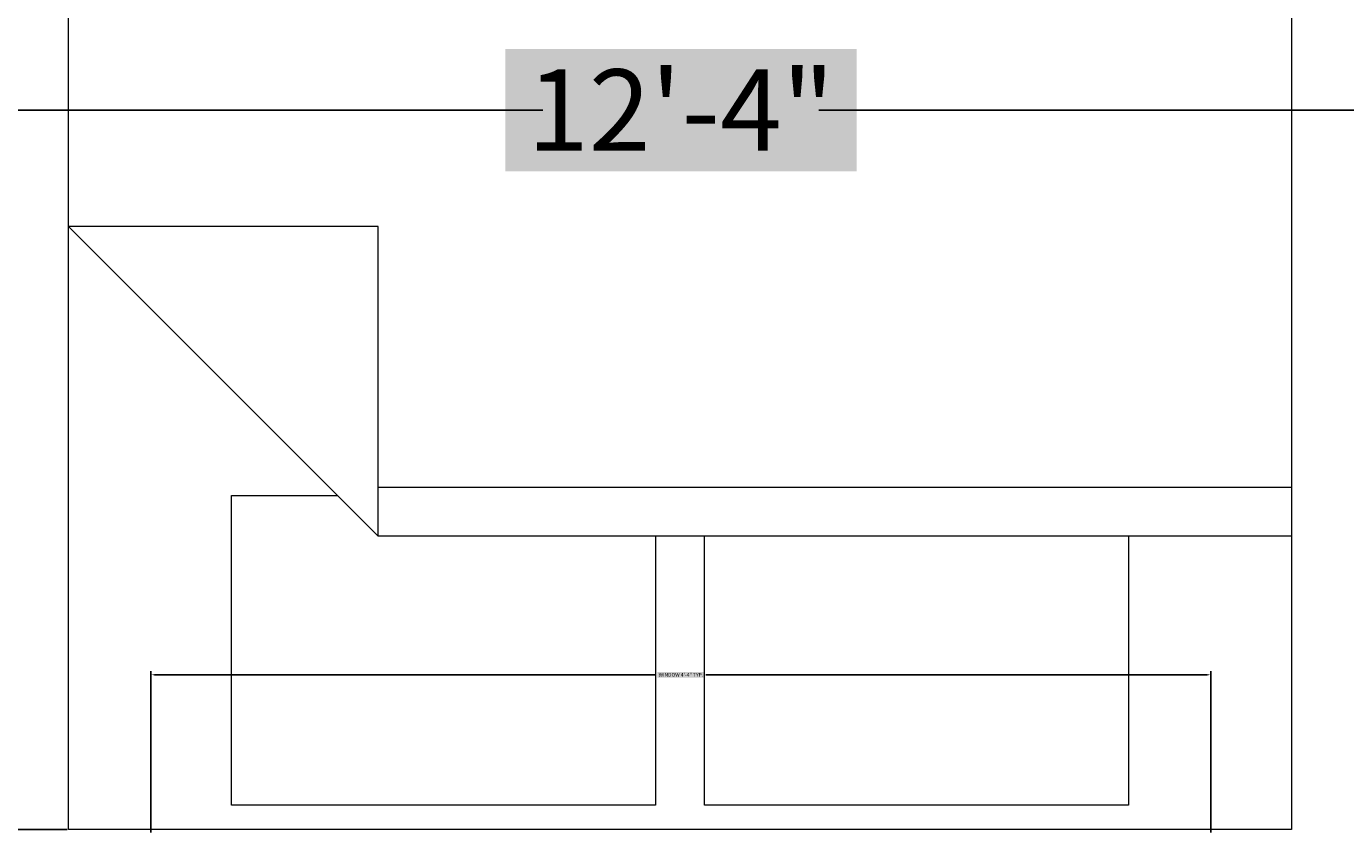
# Model space of a CAD drawing. Units: inches. Extents: x -128 to 854, y -395 to 398.
# Tile 25 of 61: x 199 to 263, y -80 to -41. Entities that reach past the tile are written whole.
import ezdxf

# ---------------------------------------------------------------- set-up
doc = ezdxf.new("R2010")
doc.units = ezdxf.units.IN
doc.header["$MEASUREMENT"] = 0
doc.layers.add('A-ANNO-DIMS', color=2, linetype='Continuous', lineweight=18)
doc.layers.add('A-FURN', color=8, linetype='Continuous', lineweight=18)
doc.styles.get("Standard").update_dxf_attribs({"font": 'arial.ttf'})
doc.dimstyles.get("Standard").update_dxf_attribs({"dimtxt": 0.18, "dimasz": 0.18, "dimexe": 0.18, "dimexo": 0.0625, "dimgap": 0.09, "dimtad": 0, "dimtih": 1, "dimtoh": 1, "dimdec": 1, "dimzin": 0, "dimdsep": 46, "dimlunit": 4, "dimtxsty": 'Standard', "dimcen": 0.09, "dimclrd": 1, "dimclre": 2, "dimclrt": 6, "dimadec": 0, "dimazin": 0, "dimtfac": 1, "dimtdec": 1, "dimtofl": 0, "dimtmove": 0, "dimatfit": 3, "dimfxl": 1, "dimtfill": 2, "dimtfillclr": 3, "dimtolj": 1, "dimtzin": 0, "dimarcsym": 0})

# ---------------------------------------------------------------- blocks, each defined once
blk = doc.blocks.new('Bed - Queen')
for p, q in [((0, -80.00003), (0, 0)), ((0, 0), (59.99999, 0)), ((59.99999, 0), (59.99999, -80.00003)), ((7.99999, -1.2), (28.79998, -1.2)), ((7.99999, -14.4), (7.99999, -1.2)), ((28.79998, -1.2), (28.79998, -14.4)), ((31.19999, -1.2), (51.99999, -1.2)), ((31.19999, -14.4), (31.19999, -1.2)), ((51.99999, -1.2), (51.99999, -16.4)), ((0, -14.4), (44.8, -14.4)), ((59.99999, -29.6), (44.8, -14.4)), ((44.8, -14.4), (44.8, -29.6)), ((44.8, -16.8), (0, -16.8)), ((51.99999, -16.4), (46.79936, -16.4)), ((44.8, -29.6), (59.99999, -29.6))]:
    blk.add_line(p, q)
blk = doc.blocks.new('*D43')
at = {"layer": 'A-ANNO-DIMS', "color": 0, "lineweight": -2, "transparency": 16777216}
for p, q in [((156.873, -80.197), (156.873, -44.559)), ((304.873, -80.197), (304.873, -44.559)), ((161.873, -44.739), (224.101, -44.739)), ((299.873, -44.739), (237.645, -44.739))]:
    blk.add_line(p, q, dxfattribs=at)
at = {"layer": 'A-ANNO-DIMS', "color": 0, "transparency": 16777216}
for points in [[(161.873, -43.906), (161.873, -45.572), (156.873, -44.739)], [(299.873, -43.906), (299.873, -45.572), (304.873, -44.739)]]:
    blk.add_solid(points, dxfattribs=at)
at = {"layer": 'Defpoints', "color": 0, "transparency": 16777216}
for p in [(304.873, -44.739), (156.873, -80.259), (304.873, -80.259)]:
    blk.add_point(p, dxfattribs=at)
at = {"layer": 'A-ANNO-DIMS', "color": 0, "transparency": 16777216, "insert": (230.873, -44.739), "char_height": 4, "attachment_point": 5, "bg_fill": 1, "box_fill_scale": 1.25, "bg_fill_color": 3, "bg_fill_transparency": 0}
blk.add_mtext('\\A1;12\'-4"', dxfattribs=at)
blk = doc.blocks.new('*D71')
at = {"layer": 'A-ANNO-DIMS', "color": 2, "lineweight": -2, "transparency": 16777216}
for p, q in [((204.873, -80.197), (204.873, -72.279)), ((256.873, -80.197), (256.873, -72.279))]:
    blk.add_line(p, q, dxfattribs=at)
at = {"layer": 'A-ANNO-DIMS', "color": 1, "lineweight": -2, "transparency": 16777216}
for p, q in [((205.053, -72.459), (229.644, -72.459)), ((256.693, -72.459), (232.102, -72.459))]:
    blk.add_line(p, q, dxfattribs=at)
at = {"layer": 'A-ANNO-DIMS', "color": 1, "transparency": 16777216}
for points in [[(205.053, -72.429), (205.053, -72.489), (204.873, -72.459)], [(256.693, -72.429), (256.693, -72.489), (256.873, -72.459)]]:
    blk.add_solid(points, dxfattribs=at)
at = {"layer": 'Defpoints', "color": 0, "transparency": 16777216}
for p in [(204.873, -72.459), (204.873, -80.259), (256.873, -80.259)]:
    blk.add_point(p, dxfattribs=at)
at = {"layer": 'A-ANNO-DIMS', "color": 6, "transparency": 16777216, "insert": (230.873, -72.459), "char_height": 0.18, "attachment_point": 5, "bg_fill": 1, "box_fill_scale": 1.25, "bg_fill_color": 3, "bg_fill_transparency": 0}
blk.add_mtext('\\A1;WINDOW 4\'-4" TYP.', dxfattribs=at)
blk = doc.blocks.new('*D77')
at = {"layer": 'A-ANNO-DIMS', "color": 2, "lineweight": -2, "transparency": 16777216}
for p, q in [((200.764, -0.056), (188.647, -0.056)), ((200.764, -80.056), (188.647, -80.056))]:
    blk.add_line(p, q, dxfattribs=at)
at = {"layer": 'A-ANNO-DIMS', "color": 1, "lineweight": -2, "transparency": 16777216}
for p, q in [((188.827, -0.236), (188.827, -39.867)), ((188.827, -79.876), (188.827, -40.245))]:
    blk.add_line(p, q, dxfattribs=at)
at = {"layer": 'A-ANNO-DIMS', "color": 1, "transparency": 16777216}
for points in [[(188.797, -0.236), (188.857, -0.236), (188.827, -0.056)], [(188.797, -79.876), (188.857, -79.876), (188.827, -80.056)]]:
    blk.add_solid(points, dxfattribs=at)
at = {"layer": 'Defpoints', "color": 0, "transparency": 16777216}
for p in [(200.827, -0.056), (188.827, -80.056), (200.827, -80.056)]:
    blk.add_point(p, dxfattribs=at)
at = {"layer": 'A-ANNO-DIMS', "color": 6, "transparency": 16777216, "insert": (188.827, -40.056), "char_height": 0.18, "attachment_point": 5, "bg_fill": 1, "box_fill_scale": 1.25, "bg_fill_color": 3, "bg_fill_transparency": 0}
blk.add_mtext('\\A1;QUEEN BED 6\'-8" TYP.', dxfattribs=at)

msp = doc.modelspace()

# ---------------------------------------------------------------- block references
at = {"layer": 'A-FURN', "rotation": 180}
msp.add_blockref('Bed - Queen', (260.827, -80.056), dxfattribs=at)

# ---------------------------------------------------------------- dimensions: what is measured, and where the dimension line sits
at = {"layer": 'A-ANNO-DIMS'}
for base, p1, p2, angle, text, picture, middle in [((188.827, -80.056), (200.827, -0.056), (200.827, -80.056), 270, 'QUEEN BED <> TYP.', '*D77', (188.827, -40.056)), ((204.873, -72.459), (256.873, -80.259), (204.873, -80.259), 180, 'WINDOW <> TYP.', '*D71', (230.873, -72.459))]:
    dim = msp.add_linear_dim(base=base, p1=p1, p2=p2, angle=angle, text=text, dimstyle='Standard', override={"dimdec": 1, "dimlfac": 1, "dimrnd": 0, "dimzin": 1, "dimdsep": 46, "dimlunit": 4, "dimfrac": 2}, dxfattribs=at)
    dim.commit()
    dim.dimension.update_dxf_attribs({"geometry": picture, "text_midpoint": middle})
dim = msp.add_linear_dim(base=(304.873, -44.739), p1=(156.873, -80.259), p2=(304.873, -80.259), dimstyle='Standard', override={"dimtxt": 4, "dimasz": 5, "dimclrd": 0, "dimclre": 0, "dimclrt": 0}, dxfattribs=at)
dim.commit()
dim.dimension.update_dxf_attribs({"geometry": '*D43', "text_midpoint": (230.873, -44.739)})

doc.saveas('drawing.dxf')
